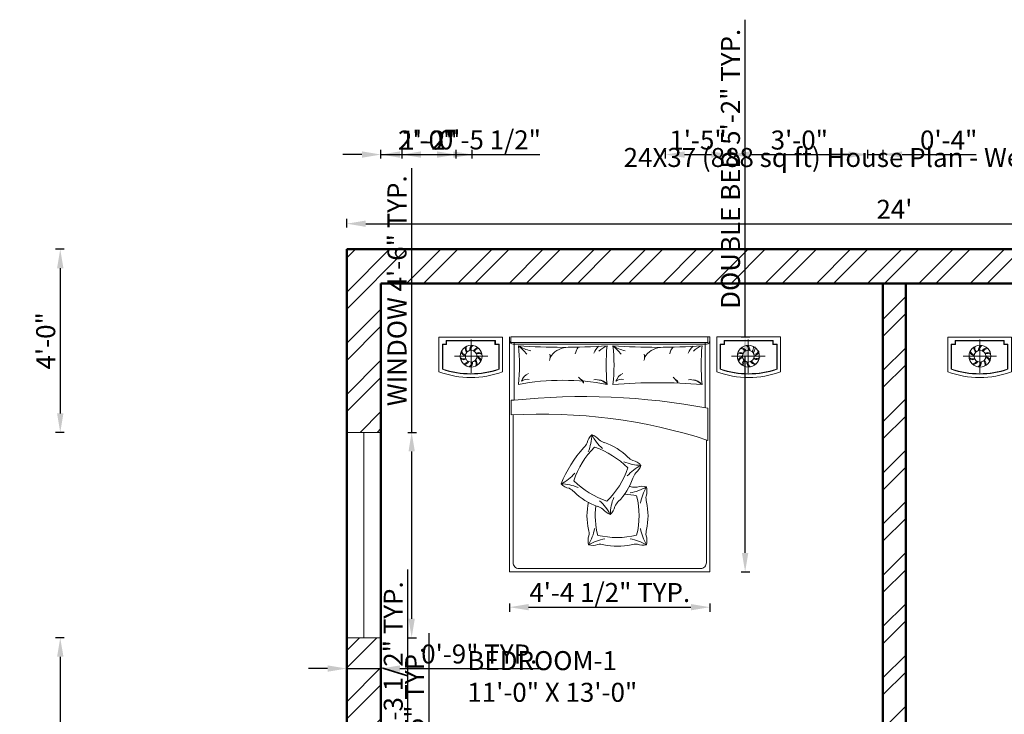
# Model space of a CAD drawing. Units: inches. Extents: x -83 to 371, y -457 to 76.
# Tile 3 of 4: x -83 to 176, y -107 to 76. Entities that reach past the tile are written whole.
import ezdxf

# ---------------------------------------------------------------- set-up
doc = ezdxf.new("R2010")
doc.units = ezdxf.units.IN
for name, color, linetype, lineweight in [('A-ANNO-DIMS', 2, 'Continuous', 18), ('A-ANNO-TEXT', 7, 'Continuous', 25), ('A-AREA-IDEN', 7, 'Continuous', 25), ('A-GLAZ', 4, 'Continuous', 18), ('A-WALL', 7, 'Continuous', 50), ('A-WALL-PATT', 252, 'Continuous', 13), ('furn', 28, 'Continuous', 18)]:
    doc.layers.add(name, color=color, linetype=linetype, lineweight=lineweight)
doc.styles.get("Standard").update_dxf_attribs({"font": 'arial.ttf'})
doc.dimstyles.new('ISO-25', dxfattribs={"dimtxt": 5, "dimasz": 5, "dimexe": 1.25, "dimexo": 0.625, "dimtad": 1, "dimlunit": 3, "dimtxsty": 'Standard', "dimcen": 2.5, "dimadec": 0, "dimazin": 0, "dimtfac": 1, "dimtmove": 0, "dimatfit": 3, "dimfxl": 1, "dimfxlon": 1, "dimarcsym": 0})

# ---------------------------------------------------------------- blocks, each defined once
blk = doc.blocks.new('*D8')
at = {"layer": 'A-ANNO-DIMS', "color": 0, "lineweight": -2, "transparency": 16777216}
for p, q in [((2.97, 21.4), (2.97, 23.65)), ((290.97, 21.4), (290.97, 23.65)), ((7.97, 22.4), (285.97, 22.4))]:
    blk.add_line(p, q, dxfattribs=at)
at = {"layer": 'A-ANNO-DIMS', "color": 0, "transparency": 16777216}
for points in [[(7.97, 23.23), (7.97, 21.56), (2.97, 22.4)], [(285.97, 23.23), (285.97, 21.56), (290.97, 22.4)]]:
    blk.add_solid(points, dxfattribs=at)
at = {"layer": 'Defpoints', "color": 0, "transparency": 16777216}
for p in [(290.97, 22.4), (2.97, 15.68), (290.97, 15.68)]:
    blk.add_point(p, dxfattribs=at)
at = {"layer": 'A-ANNO-DIMS', "color": 0, "transparency": 16777216, "insert": (146.97, 25.53), "char_height": 5, "attachment_point": 5}
blk.add_mtext("24'", dxfattribs=at)
blk = doc.blocks.new('BED-DOUBLE')
for p, q in [((0.91, 59.91), (51.75, 59.91)), ((1.17, 60.37), (1.17, 45.16)), ((51.46, 60.37), (51.46, 43.19))]:
    blk.add_line(p, q)
for points in [[(0, 61.8), (0, 0), (52.66, 0), (52.66, 61.8)], [(52.17, 61.8), (52.17, 60.37), (0.3, 60.37), (0.3, 61.8), (52.66, 61.8)]]:
    blk.add_lwpolyline(points)
for points in [[(2.33, 49.32, 0.058596), (2.33, 59.5, 0.036889), (25.64, 59.5, 0.052163), (25.64, 49.32, 0.093111)], [(27.16, 49.32, 0.058596), (27.16, 59.5, 0.036648), (50.62, 59.5, 0.052163), (50.62, 49.32, 0.036967)], [(0.46, 45.16), (1.17, 45.16, -0.072944), (52.17, 43.04), (52.17, 34.6, 0.092568), (0.46, 41.29)]]:
    blk.add_lwpolyline(points, format="xyb", close=True)
for points in [[(0.91, 41.32), (0.91, 2.43, 0.414214), (2.43, 0.91), (50.23, 0.91, 0.414214), (51.75, 2.43), (51.75, 34.75)], [(20.68, 31.62, 0.091296), (21.61, 36.08, 0.091296), (24.41, 32.49, 0.091296)], [(16.91, 24, 0.111006), (25.6, 18.59, 0.119549), (31.09, 27.39, 0.107813), (22.42, 32.82)], [(22.37, 32.81, 0.121865), (16.91, 24, 0.121865)], [(30.07, 28.97, 0.091296), (34.52, 28.03, 0.091296), (30.93, 25.24, 0.091296)], [(18.01, 22.22, 0.091296), (13.56, 23.16, 0.091296), (17.15, 25.96, 0.091296)], [(26.47, 15.11, 0.159461), (27.65, 17.2, -0.076283), (28.59, 18.51, 0.115075), (32.41, 24.64, -0.076283), (33.17, 26.05, 0.159461), (34.52, 28.03)], [(31.71, 20.79, 0.091296), (35.99, 22.35, 0.091296), (34.42, 18.08, 0.091296)], [(35.99, 7.13, 0.159461), (35.88, 9.53, -0.076283), (35.99, 11.13, 0.115075), (35.99, 18.36, -0.076283), (35.88, 19.96, 0.159461), (35.99, 22.35)], [(23.17, 9.62, 0.111006), (33.41, 9.63, 0.119549), (33.41, 19.99, 0.033212), (30.26, 20.47)], [(27.4, 19.57, 0.091296), (26.47, 15.11, 0.091296), (23.67, 18.7)], [(25.05, 8.69, 0.091296), (20.77, 7.13, 0.091296), (22.34, 11.41, 0.091296)], [(34.42, 11.41, 0.091296), (35.99, 7.13, 0.091296), (31.71, 8.69)]]:
    blk.add_lwpolyline(points, format="xyb")
for centre, radius, start, end in [((0.91, 60.83), 0.913, 180, 270), ((51.75, 60.83), 0.913, 270, 0), ((7.74, 68), 10.08, 237.5379, 257.5233), ((-5.29, 49.98), 12.19, 36.4935, 51.2792), ((8.15, 56.6), 2.53, 335.8927, 16.1192), ((15.48, 53.46), 5.64, 96.6849, 148.3182), ((21.18, 56.67), 3.96, 141.8174, 169.8987), ((26.19, 56.11), 4.26, 130.5354, 160.3558), ((28.84, 52.52), 7.67, 114.6457, 134.1585), ((19.53, 49.98), 12.19, 36.4935, 51.2792), ((32.57, 68), 10.08, 237.5379, 257.5233), ((32.98, 56.6), 2.53, 335.8927, 16.1192), ((40.3, 53.46), 5.64, 96.6849, 148.3182), ((46.01, 56.67), 3.96, 141.8174, 169.8987), ((51.01, 56.11), 4.26, 130.5354, 160.3558), ((53.67, 52.52), 7.67, 114.6457, 134.1585), ((6.34, 49.09), 3.38, 114.2916, 160.9896), ((31.17, 49.09), 3.38, 114.2916, 160.9896), ((4.59, 48.38), 2.31, 76.4823, 128.5563), ((9.19, 42.25), 12.71, 36.2085, 45.0849), ((18.6, 49.75), 0.853, 353.7543, 77.2187), ((22.67, 46.41), 4.16, 44.406, 96.8342), ((23.45, 47.86), 2.64, 33.6349, 90.8456), ((29.41, 48.38), 2.31, 76.4823, 128.5563), ((34.02, 42.25), 12.71, 36.2085, 45.0849), ((43.42, 49.75), 0.853, 353.7543, 77.2187), ((47.5, 46.41), 4.16, 44.406, 96.8342), ((48.27, 47.86), 2.64, 33.6349, 90.8456), ((15.72, 36.39), 5.29, 315.5854, 333.0343), ((24.21, 33.23), 3.86, 132.4658, 168.7065), ((20.58, 32.5), 3.72, 37.2937, 74.0973), ((26.71, 38.99), 5.29, 233.2983, 250.7472), ((19.89, 18.93), 15.91, 45.1307, 71.3884), ((44.41, 10.55), 33.33, 138.3818, 157.7644), ((34.79, 33.99), 5.29, 225.7718, 243.2208), ((31.77, 25.77), 3.56, 39.4726, 79.6505), ((16.39, 25.78), 3.86, 222.6522, 258.8929), ((13.27, 17.27), 5.29, 45.7718, 63.2208), ((28.18, 32.33), 15.91, 225.1307, 251.3884), ((28.38, 6.89), 15.91, 77.0576, 78.7033), ((33.07, 27.55), 5.29, 257.6988, 275.1477), ((34.85, 18.98), 3.56, 71.3996, 111.5774), ((36.26, 14.74), 15.91, 166.8711, 193.1289), ((44.1, 14.85), 21.58, 173.1956, 194.0284), ((21.36, 12.27), 5.29, 53.2983, 70.7472), ((27.96, 19.27), 4.41, 218.7754, 250.3571), ((15.61, 9.99), 5.29, 355.0387, 12.4877), ((24.48, 8.17), 3.86, 159.3666, 195.6073), ((21.79, 10.85), 3.86, 254.5791, 290.8198), ((23.64, 1.98), 5.29, 77.6988, 95.1477), ((28.33, 22.65), 15.91, 257.0576, 283.3153), ((33.15, 2.01), 5.29, 85.2252, 102.6741), ((35.05, 11.45), 4.41, 250.7023, 282.284)]:
    blk.add_arc(centre, radius, start, end)
blk = doc.blocks.new('NIGHTSTAND-L')
for p, q in [((8.46, 1.22), (8.46, 10)), ((4.07, 5.61), (12.85, 5.61))]:
    blk.add_line(p, q)
blk.add_lwpolyline([(0, 1.52), (0, 10.65), (16.74, 10.65), (16.74, 1.52, -0.181818)], format="xyb", close=True)
for points in [[(1.92, 9.74), (1.92, 8.74), (0.91, 8.74)], [(2.01, 9.74), (2.01, 8.65), (0.91, 8.65)], [(1.92, 9.74), (14.83, 9.74)], [(1.92, 9.65), (14.83, 9.65)], [(14.73, 9.74), (14.73, 8.65), (15.83, 8.65)], [(14.83, 9.74), (14.83, 8.74), (15.83, 8.74)]]:
    blk.add_lwpolyline(points)
for points in [[(15.83, 8.74), (15.83, 2.16, -0.167087), (0.91, 2.16), (0.91, 8.74)], [(15.74, 8.74), (15.74, 2.22, -0.165559), (1, 2.22), (1, 8.74)]]:
    blk.add_lwpolyline(points, format="xyb")
for radius in [2.87, 1.55]:
    blk.add_circle((8.46, 5.61), radius)
for centre, radius, start, end in [((8.71, 7.76), 1.84, 172.17, 218.4897), ((8.53, 7.72), 1.41, 160.3002, 220.538), ((9.93, 7.2), 1.84, 136.17, 182.4897), ((9.76, 7.27), 1.41, 124.3002, 184.538), ((10.58, 6.04), 1.84, 100.17, 146.4897), ((6.48, 6.34), 1.41, 232.3002, 292.538), ((7.4, 7.5), 1.84, 208.17, 254.4897), ((7.28, 7.36), 1.41, 196.3002, 256.538), ((10.49, 6.19), 1.41, 88.3002, 148.538), ((10.42, 4.71), 1.84, 64.17, 110.4897), ((10.44, 4.89), 1.41, 52.3002, 112.538), ((9.64, 3.86), 1.41, 16.3002, 76.538), ((9.52, 3.73), 1.84, 28.17, 74.4897), ((6.49, 6.52), 1.84, 244.17, 290.4897), ((6.43, 5.03), 1.41, 268.3002, 328.538), ((6.34, 5.19), 1.84, 280.17, 326.4897), ((7.16, 3.95), 1.41, 304.3002, 4.538), ((6.99, 4.02), 1.84, 316.17, 2.4897), ((8.38, 3.51), 1.41, 340.3002, 40.538), ((8.2, 3.47), 1.84, 352.17, 38.4897)]:
    blk.add_arc(centre, radius, start, end)
blk = doc.blocks.new('NIGHTSTAND-R')
for p, q in [((8.28, 1.22), (8.28, 10)), ((12.67, 5.61), (3.89, 5.61))]:
    blk.add_line(p, q)
blk.add_lwpolyline([(16.74, 1.52), (16.74, 10.65), (0, 10.65), (0, 1.52, 0.181818)], format="xyb", close=True)
for points in [[(1.92, 9.74), (1.92, 8.74), (0.91, 8.74)], [(2.01, 9.74), (2.01, 8.65), (0.91, 8.65)], [(14.82, 9.74), (1.92, 9.74)], [(14.82, 9.65), (1.92, 9.65)], [(14.73, 9.74), (14.73, 8.65), (15.83, 8.65)], [(14.82, 9.74), (14.82, 8.74), (15.83, 8.74)]]:
    blk.add_lwpolyline(points)
for points in [[(0.91, 8.74), (0.91, 2.16, 0.167087), (15.83, 2.16), (15.83, 8.74)], [(1, 8.74), (1, 2.22, 0.165559), (15.74, 2.22), (15.74, 8.74)]]:
    blk.add_lwpolyline(points, format="xyb")
for radius in [2.87, 1.55]:
    blk.add_circle((8.28, 5.61), radius)
for centre, radius, start, end in [((6.16, 6.03), 1.84, 33.5103, 79.83), ((6.99, 7.27), 1.41, 355.462, 55.6998), ((6.82, 7.2), 1.84, 357.5103, 43.83), ((8.21, 7.72), 1.41, 319.462, 19.6998), ((8.24, 7.84), 1.84, 321.5103, 7.83), ((6.3, 4.89), 1.41, 67.462, 127.6998), ((6.32, 4.7), 1.84, 69.5103, 115.83), ((7.23, 3.72), 1.84, 105.5103, 151.83), ((7.11, 3.86), 1.41, 103.462, 163.6998), ((6.26, 6.19), 1.41, 31.462, 91.6998), ((10.48, 6.41), 1.41, 247.462, 307.6998), ((9.67, 7.44), 1.41, 283.462, 343.6998), ((9.55, 7.58), 1.84, 285.5103, 331.83), ((8.54, 3.46), 1.84, 141.5103, 187.83), ((8.36, 3.5), 1.41, 139.462, 199.6998), ((9.75, 4.02), 1.84, 177.5103, 223.83), ((9.58, 3.95), 1.41, 175.462, 235.6998), ((10.41, 5.19), 1.84, 213.5103, 259.83), ((10.31, 5.03), 1.41, 211.462, 271.6998), ((10.46, 6.59), 1.84, 249.5103, 295.83)]:
    blk.add_arc(centre, radius, start, end)
blk = doc.blocks.new('WIN-54IN')
blk.add_line((4.5, 54), (4.5, 0))
blk.add_lwpolyline([(0, 54), (9, 54), (9, 0), (0, 0)], close=True)
blk = doc.blocks.new('*D18')
at = {"layer": 'A-ANNO-DIMS', "color": 0, "lineweight": -2, "transparency": 16777216}
for p, q in [((20.04, -32.5), (20.04, 37.02)), ((19.04, -32.5), (21.29, -32.5)), ((20.04, -81.5), (20.04, -37.5)), ((19.04, -86.5), (21.29, -86.5))]:
    blk.add_line(p, q, dxfattribs=at)
at = {"layer": 'A-ANNO-DIMS', "color": 0, "transparency": 16777216}
for points in [[(19.21, -37.5), (20.87, -37.5), (20.04, -32.5)], [(19.21, -81.5), (20.87, -81.5), (20.04, -86.5)]]:
    blk.add_solid(points, dxfattribs=at)
at = {"layer": 'Defpoints', "color": 0, "transparency": 16777216}
for p in [(11.94, -32.5), (20.04, -32.5), (11.94, -86.5)]:
    blk.add_point(p, dxfattribs=at)
at = {"layer": 'A-ANNO-DIMS', "color": 0, "transparency": 16777216, "insert": (16.83, 4.76), "char_height": 5, "attachment_point": 5, "rotation": 90}
blk.add_mtext('WINDOW 4\'-6" TYP.', dxfattribs=at)
blk = doc.blocks.new('*D19')
at = {"layer": 'A-ANNO-DIMS', "color": 0, "lineweight": -2, "transparency": 16777216}
for p, q in [((-2.06, -94.6), (-7.06, -94.6)), ((2.94, -93.6), (2.94, -95.85)), ((2.94, -94.6), (11.94, -94.6)), ((11.94, -93.6), (11.94, -95.85)), ((16.94, -94.6), (53.67, -94.6))]:
    blk.add_line(p, q, dxfattribs=at)
at = {"layer": 'A-ANNO-DIMS', "color": 0, "transparency": 16777216}
for points in [[(-2.06, -93.77), (-2.06, -95.43), (2.94, -94.6)], [(16.94, -93.77), (16.94, -95.43), (11.94, -94.6)]]:
    blk.add_solid(points, dxfattribs=at)
at = {"layer": 'Defpoints', "color": 0, "transparency": 16777216}
for p in [(2.94, -86.5), (11.94, -86.5), (11.94, -94.6)]:
    blk.add_point(p, dxfattribs=at)
at = {"layer": 'A-ANNO-DIMS', "color": 0, "transparency": 16777216, "insert": (37.8, -91.42), "char_height": 5, "attachment_point": 5}
blk.add_mtext('0\'-9" TYP.', dxfattribs=at)
blk = doc.blocks.new('*D22')
at = {"layer": 'A-ANNO-DIMS', "color": 0, "lineweight": -2, "transparency": 16777216}
for p, q in [((107.72, -7.39), (107.72, 76.05)), ((106.72, -7.39), (108.97, -7.39)), ((107.72, -64.19), (107.72, -12.39)), ((106.72, -69.19), (108.97, -69.19))]:
    blk.add_line(p, q, dxfattribs=at)
at = {"layer": 'A-ANNO-DIMS', "color": 0, "transparency": 16777216}
for points in [[(106.88, -12.39), (108.55, -12.39), (107.72, -7.39)], [(106.88, -64.19), (108.55, -64.19), (107.72, -69.19)]]:
    blk.add_solid(points, dxfattribs=at)
at = {"layer": 'Defpoints', "color": 0, "transparency": 16777216}
for p in [(98.45, -7.39), (107.72, -7.39), (98.45, -69.19)]:
    blk.add_point(p, dxfattribs=at)
at = {"layer": 'A-ANNO-DIMS', "color": 0, "transparency": 16777216, "insert": (104.51, 36.83), "char_height": 5, "attachment_point": 5, "rotation": 90}
blk.add_mtext('DOUBLE BED 5\'-2" TYP.', dxfattribs=at)
blk = doc.blocks.new('*D23')
at = {"layer": 'A-ANNO-DIMS', "color": 0, "lineweight": -2, "transparency": 16777216}
for p, q in [((45.78, -77.46), (45.78, -79.71)), ((98.45, -77.46), (98.45, -79.71)), ((50.78, -78.46), (93.45, -78.46))]:
    blk.add_line(p, q, dxfattribs=at)
at = {"layer": 'A-ANNO-DIMS', "color": 0, "transparency": 16777216}
for points in [[(50.78, -77.63), (50.78, -79.29), (45.78, -78.46)], [(93.45, -77.63), (93.45, -79.29), (98.45, -78.46)]]:
    blk.add_solid(points, dxfattribs=at)
at = {"layer": 'Defpoints', "color": 0, "transparency": 16777216}
for p in [(45.78, -69.19), (98.45, -69.19), (98.45, -78.46)]:
    blk.add_point(p, dxfattribs=at)
at = {"layer": 'A-ANNO-DIMS', "color": 0, "transparency": 16777216, "insert": (72.12, -75.25), "char_height": 5, "attachment_point": 5}
blk.add_mtext('4\'-4 1/2" TYP.', dxfattribs=at)
blk = doc.blocks.new('*D30')
at = {"layer": 'A-ANNO-DIMS', "color": 0, "lineweight": -2, "transparency": 16777216}
for p, q in [((24.67, -178.88), (24.67, -85.32)), ((24.53, -183.88), (25.92, -183.88)), ((24.67, -188.98), (24.67, -183.88)), ((24.53, -188.98), (25.92, -188.98)), ((24.67, -193.98), (24.67, -198.98))]:
    blk.add_line(p, q, dxfattribs=at)
at = {"layer": 'A-ANNO-DIMS', "color": 0, "transparency": 16777216}
for points in [[(23.83, -178.88), (25.5, -178.88), (24.67, -183.88)], [(23.83, -193.98), (25.5, -193.98), (24.67, -188.98)]]:
    blk.add_solid(points, dxfattribs=at)
at = {"layer": 'Defpoints', "color": 0, "transparency": 16777216}
for p in [(23.9, -183.88), (24.67, -183.88), (23.9, -188.98)]:
    blk.add_point(p, dxfattribs=at)
at = {"layer": 'A-ANNO-DIMS', "color": 0, "transparency": 16777216, "insert": (21.46, -129.6), "char_height": 5, "attachment_point": 5, "rotation": 90}
blk.add_mtext('LARGE BURNER 0\'-5" TYP.', dxfattribs=at)
blk = doc.blocks.new('*D32')
at = {"layer": 'A-ANNO-DIMS', "color": 0, "lineweight": -2, "transparency": 16777216}
for p, q in [((19.06, -173.23), (19.06, -68.59)), ((19.06, -178.23), (17.81, -178.23)), ((19.06, -181.8), (19.06, -178.23)), ((19.06, -181.8), (17.81, -181.8)), ((19.06, -186.8), (19.06, -191.8))]:
    blk.add_line(p, q, dxfattribs=at)
at = {"layer": 'A-ANNO-DIMS', "color": 0, "transparency": 16777216}
for points in [[(18.23, -173.23), (19.9, -173.23), (19.06, -178.23)], [(18.23, -186.8), (19.9, -186.8), (19.06, -181.8)]]:
    blk.add_solid(points, dxfattribs=at)
at = {"layer": 'Defpoints', "color": 0, "transparency": 16777216}
for p in [(19.06, -178.23), (19.6, -178.23), (19.6, -181.8)]:
    blk.add_point(p, dxfattribs=at)
at = {"layer": 'A-ANNO-DIMS', "color": 0, "transparency": 16777216, "insert": (15.85, -118.41), "char_height": 5, "attachment_point": 5, "rotation": 90}
blk.add_mtext('SMALL BURNER 0\'-3 1/2" TYP.', dxfattribs=at)
blk = doc.blocks.new('*D38')
at = {"layer": 'A-ANNO-DIMS', "color": 0, "lineweight": -2, "transparency": 16777216}
for p, q in [((-71.36, 15.68), (-73.61, 15.68)), ((-72.36, 10.68), (-72.36, -27.5)), ((-71.36, -32.5), (-73.61, -32.5))]:
    blk.add_line(p, q, dxfattribs=at)
at = {"layer": 'A-ANNO-DIMS', "color": 0, "transparency": 16777216}
for points in [[(-73.19, 10.68), (-71.52, 10.68), (-72.36, 15.68)], [(-73.19, -27.5), (-71.52, -27.5), (-72.36, -32.5)]]:
    blk.add_solid(points, dxfattribs=at)
at = {"layer": 'Defpoints', "color": 0, "transparency": 16777216}
for p in [(2.97, 15.68), (-72.36, -32.5), (2.94, -32.5)]:
    blk.add_point(p, dxfattribs=at)
at = {"layer": 'A-ANNO-DIMS', "color": 0, "transparency": 16777216, "insert": (-75.54, -8.41), "char_height": 5, "attachment_point": 5, "rotation": 90}
blk.add_mtext('4\'-0"', dxfattribs=at)
blk = doc.blocks.new('*D39')
at = {"layer": 'A-ANNO-DIMS', "color": 0, "lineweight": -2, "transparency": 16777216}
for p, q in [((-71.36, -86.5), (-73.61, -86.5)), ((-72.36, -91.5), (-72.36, -163.99)), ((-71.36, -168.99), (-73.61, -168.99))]:
    blk.add_line(p, q, dxfattribs=at)
at = {"layer": 'A-ANNO-DIMS', "color": 0, "transparency": 16777216}
for points in [[(-73.19, -91.5), (-71.52, -91.5), (-72.36, -86.5)], [(-73.19, -163.99), (-71.52, -163.99), (-72.36, -168.99)]]:
    blk.add_solid(points, dxfattribs=at)
at = {"layer": 'Defpoints', "color": 0, "transparency": 16777216}
for p in [(2.94, -86.5), (-72.36, -168.99), (3.06, -168.99)]:
    blk.add_point(p, dxfattribs=at)
at = {"layer": 'A-ANNO-DIMS', "color": 0, "transparency": 16777216, "insert": (-75.57, -127.74), "char_height": 5, "attachment_point": 5, "rotation": 90}
blk.add_mtext('6\'-10 1/2"', dxfattribs=at)
blk = doc.blocks.new('*D45')
at = {"layer": 'A-ANNO-DIMS', "color": 0, "lineweight": -2, "transparency": 16777216}
for p, q in [((143.97, -455.2), (143.97, -457.45)), ((149.97, -455.2), (149.97, -457.45)), ((138.97, -456.2), (133.97, -456.2)), ((143.97, -456.2), (149.97, -456.2)), ((154.97, -456.2), (174.51, -456.2))]:
    blk.add_line(p, q, dxfattribs=at)
at = {"layer": 'A-ANNO-DIMS', "color": 0, "transparency": 16777216}
for points in [[(138.97, -455.37), (138.97, -457.03), (143.97, -456.2)], [(154.97, -455.37), (154.97, -457.03), (149.97, -456.2)]]:
    blk.add_solid(points, dxfattribs=at)
at = {"layer": 'Defpoints', "color": 0, "transparency": 16777216}
for p in [(143.97, 6.68), (149.97, 6.68), (149.97, -456.2)]:
    blk.add_point(p, dxfattribs=at)
at = {"layer": 'A-ANNO-DIMS', "color": 0, "transparency": 16777216, "insert": (167.24, -453.02), "char_height": 5, "attachment_point": 5}
blk.add_mtext('0\'-6"', dxfattribs=at)
blk = doc.blocks.new('*D46')
at = {"layer": 'A-ANNO-DIMS', "color": 0, "lineweight": -2, "transparency": 16777216}
for p, q in [((103.97, 39.58), (103.97, 41.83)), ((139.97, 39.58), (139.97, 41.83)), ((108.97, 40.58), (134.97, 40.58))]:
    blk.add_line(p, q, dxfattribs=at)
at = {"layer": 'A-ANNO-DIMS', "color": 0, "transparency": 16777216}
for points in [[(108.97, 41.41), (108.97, 39.74), (103.97, 40.58)], [(134.97, 41.41), (134.97, 39.74), (139.97, 40.58)]]:
    blk.add_solid(points, dxfattribs=at)
at = {"layer": 'Defpoints', "color": 0, "transparency": 16777216}
for p in [(139.97, 40.58), (103.97, -149.32), (139.97, -149.32)]:
    blk.add_point(p, dxfattribs=at)
at = {"layer": 'A-ANNO-DIMS', "color": 0, "transparency": 16777216, "insert": (121.97, 43.75), "char_height": 5, "attachment_point": 5}
blk.add_mtext('3\'-0"', dxfattribs=at)
blk = doc.blocks.new('*D47')
at = {"layer": 'A-ANNO-DIMS', "color": 0, "lineweight": -2, "transparency": 16777216}
for p, q in [((139.97, 39.58), (139.97, 41.83)), ((143.97, 39.58), (143.97, 41.83)), ((134.97, 40.58), (129.97, 40.58)), ((139.97, 40.58), (143.97, 40.58)), ((148.97, 40.58), (168.51, 40.58))]:
    blk.add_line(p, q, dxfattribs=at)
at = {"layer": 'A-ANNO-DIMS', "color": 0, "transparency": 16777216}
for points in [[(134.97, 41.41), (134.97, 39.74), (139.97, 40.58)], [(148.97, 41.41), (148.97, 39.74), (143.97, 40.58)]]:
    blk.add_solid(points, dxfattribs=at)
at = {"layer": 'Defpoints', "color": 0, "transparency": 16777216}
for p in [(143.97, 40.58), (139.97, -149.32), (143.97, -149.32)]:
    blk.add_point(p, dxfattribs=at)
at = {"layer": 'A-ANNO-DIMS', "color": 0, "transparency": 16777216, "insert": (161.24, 43.75), "char_height": 5, "attachment_point": 5}
blk.add_mtext('0\'-4"', dxfattribs=at)
blk = doc.blocks.new('*D58')
at = {"layer": 'A-ANNO-DIMS', "color": 0, "lineweight": -2, "transparency": 16777216}
for p, q in [((11.97, 39.58), (11.97, 41.83)), ((35.97, 39.58), (35.97, 41.83)), ((16.97, 40.58), (30.97, 40.58))]:
    blk.add_line(p, q, dxfattribs=at)
at = {"layer": 'A-ANNO-DIMS', "color": 0, "transparency": 16777216}
for points in [[(16.97, 41.41), (16.97, 39.74), (11.97, 40.58)], [(30.97, 41.41), (30.97, 39.74), (35.97, 40.58)]]:
    blk.add_solid(points, dxfattribs=at)
at = {"layer": 'Defpoints', "color": 0, "transparency": 16777216}
for p in [(35.97, 40.58), (11.97, -155.32), (35.97, -155.32)]:
    blk.add_point(p, dxfattribs=at)
at = {"layer": 'A-ANNO-DIMS', "color": 0, "transparency": 16777216, "insert": (23.97, 43.75), "char_height": 5, "attachment_point": 5}
blk.add_mtext('2\'-0"', dxfattribs=at)
blk = doc.blocks.new('*D59')
at = {"layer": 'A-ANNO-DIMS', "color": 0, "lineweight": -2, "transparency": 16777216}
for p, q in [((17.51, 39.58), (17.51, 41.83)), ((31.73, 39.58), (31.73, 41.83)), ((22.51, 40.58), (26.73, 40.58))]:
    blk.add_line(p, q, dxfattribs=at)
at = {"layer": 'A-ANNO-DIMS', "color": 0, "transparency": 16777216}
for points in [[(22.51, 41.41), (22.51, 39.74), (17.51, 40.58)], [(26.73, 41.41), (26.73, 39.74), (31.73, 40.58)]]:
    blk.add_solid(points, dxfattribs=at)
at = {"layer": 'Defpoints', "color": 0, "transparency": 16777216}
for p in [(31.73, 40.58), (17.51, -176.2), (31.73, -176.2)]:
    blk.add_point(p, dxfattribs=at)
at = {"layer": 'A-ANNO-DIMS', "color": 0, "transparency": 16777216, "insert": (24.62, 43.71), "char_height": 5, "attachment_point": 5}
blk.add_mtext('1\'-2"', dxfattribs=at)
blk = doc.blocks.new('*D65')
at = {"layer": 'A-ANNO-DIMS', "color": 0, "lineweight": -2, "transparency": 16777216}
for p, q in [((86.8, 39.58), (86.8, 41.83)), ((103.87, 39.58), (103.87, 41.83)), ((91.8, 40.58), (98.87, 40.58))]:
    blk.add_line(p, q, dxfattribs=at)
at = {"layer": 'A-ANNO-DIMS', "color": 0, "transparency": 16777216}
for points in [[(91.8, 41.41), (91.8, 39.74), (86.8, 40.58)], [(98.87, 41.41), (98.87, 39.74), (103.87, 40.58)]]:
    blk.add_solid(points, dxfattribs=at)
at = {"layer": 'Defpoints', "color": 0, "transparency": 16777216}
for p in [(103.87, 40.58), (103.87, -209.32), (86.8, -211.22)]:
    blk.add_point(p, dxfattribs=at)
at = {"layer": 'A-ANNO-DIMS', "color": 0, "transparency": 16777216, "insert": (95.33, 43.75), "char_height": 5, "attachment_point": 5}
blk.add_mtext('1\'-5"', dxfattribs=at)
blk = doc.blocks.new('*D67')
at = {"layer": 'A-ANNO-DIMS', "color": 0, "lineweight": -2, "transparency": 16777216}
for p, q in [((11.97, 39.58), (11.97, 41.83)), ((17.51, 39.58), (17.51, 41.83)), ((6.97, 40.58), (1.97, 40.58)), ((11.97, 40.58), (17.51, 40.58)), ((22.51, 40.58), (53.7, 40.58))]:
    blk.add_line(p, q, dxfattribs=at)
at = {"layer": 'A-ANNO-DIMS', "color": 0, "transparency": 16777216}
for points in [[(6.97, 41.41), (6.97, 39.74), (11.97, 40.58)], [(22.51, 41.41), (22.51, 39.74), (17.51, 40.58)]]:
    blk.add_solid(points, dxfattribs=at)
at = {"layer": 'Defpoints', "color": 0, "transparency": 16777216}
for p in [(17.51, 40.58), (11.97, -155.32), (17.51, -176.2)]:
    blk.add_point(p, dxfattribs=at)
at = {"layer": 'A-ANNO-DIMS', "color": 0, "transparency": 16777216, "insert": (40.61, 43.79), "char_height": 5, "attachment_point": 5}
blk.add_mtext('0\'-5 1/2"', dxfattribs=at)

msp = doc.modelspace()

# ---------------------------------------------------------------- hatches: boundary and pattern name
at = {"layer": 'A-WALL-PATT'}
h = msp.add_hatch(dxfattribs=at)
h.set_pattern_fill('ANSI32', color=256)
h.set_pattern_definition([(45, (-445.966, 5e-14), (-6.73519, 6.73519), []), (45, (-441.476, 5e-14), (-6.73519, 6.73519), [])])
h.paths.add_polyline_path([(147.969, -419.325), (11.969, -419.325), (11.969, -408.128), (2.969, -408.128), (2.969, -428.325), (147.969, -428.325)])
h.paths.add_polyline_path([(290.969, -408.128), (281.969, -408.128), (281.969, -419.325), (197.969, -419.325), (197.969, -428.325), (290.969, -428.325)])
h.paths.add_polyline_path([(203.969, -374.325), (207.969, -374.325), (207.969, -368.325), (203.969, -368.325), (203.969, -279.294), (197.969, -279.294), (197.969, -317.37), (194.142, -317.37), (194.142, -317.678), (194.142, -323.37), (197.969, -323.37), (197.969, -374.325), (197.969, -419.325), (203.969, -419.325)])
h.paths.add_polyline_path([(290.969, -249.793), (281.969, -249.793), (281.969, -390.128), (290.969, -390.128)])
h.paths.add_polyline_path([(149.969, -323.37), (157.969, -323.37), (157.969, -317.37), (149.969, -317.37), (149.969, -279.294), (143.969, -279.294), (143.969, -371.325), (140.142, -371.325), (140.142, -371.632), (140.142, -377.325), (143.969, -377.325), (149.969, -377.325)])
h.paths.add_polyline_path([(103.969, -371.325), (11.969, -371.325), (11.969, -377.325), (103.969, -377.325)])
h.paths.add_polyline_path([(11.969, -328.391), (3.855, -328.391), (3.855, -274.391), (11.969, -274.391), (11.969, -222.986), (2.969, -222.986), (2.969, -390.128), (11.969, -390.128)])
h.paths.add_polyline_path([(149.969, -233.325), (143.969, -233.325), (11.969, -233.325), (11.969, -239.325), (143.969, -239.325), (143.969, -243.294), (144.688, -243.294), (149.969, -243.294)])
h.paths.add_polyline_path([(11.969, -86.501), (2.969, -86.501), (2.969, -168.986), (11.969, -168.986)])
h.paths.add_polyline_path([(103.969, -149.325), (11.969, -149.325), (11.969, -155.325), (103.969, -155.325)])
h.paths.add_polyline_path([(149.969, 6.675), (143.969, 6.675), (143.969, -149.325), (139.969, -149.325), (139.969, -155.325), (153.969, -155.325), (153.969, -149.325), (149.969, -149.325)])
h.paths.add_polyline_path([(281.969, -149.325), (189.973, -149.325, -0.0041567), (189.978, -149.923), (189.978, -155.325), (281.969, -155.325)])
h.paths.add_polyline_path([(290.969, -90.886), (281.969, -90.886), (281.969, -195.793), (290.969, -195.793)])
h.paths.add_polyline_path([(290.969, 15.675), (2.969, 15.675), (2.969, -32.501), (11.969, -32.501), (11.969, 6.675), (281.969, 6.675), (281.969, -36.886), (290.969, -36.886)])

# ---------------------------------------------------------------- linework, layer by layer
at = {"layer": 'A-WALL'}
for p, q in [((2.969, 15.675), (290.969, 15.675)), ((2.969, -428.325), (2.969, 15.675)), ((11.969, 6.675), (281.969, 6.675)), ((11.969, -419.325), (11.969, 6.675)), ((143.969, -149.325), (143.969, 6.675)), ((149.969, -149.325), (149.969, 6.675))]:
    msp.add_line(p, q, dxfattribs=at)

# ---------------------------------------------------------------- block references
at = {"layer": 'A-GLAZ'}
msp.add_blockref('WIN-54IN', (2.938, -86.5), dxfattribs=at)
at = {"layer": 'furn'}
for name, p in [('NIGHTSTAND-L', (27.215, -18.053)), ('BED-DOUBLE', (45.785, -69.19)), ('NIGHTSTAND-R', (100.275, -18.05)), ('NIGHTSTAND-L', (161.006, -18.053))]:
    msp.add_blockref(name, p, dxfattribs=at)

# ---------------------------------------------------------------- texts
at = {"layer": 'A-ANNO-TEXT', "insert": (75.772, 42.316), "char_height": 5, "attachment_point": 1}
msp.add_mtext_dynamic_manual_height_columns('24X37 (888 sq ft) House Plan - West Face - FP1323', width=296.42101, gutter_width=12.5, heights=[0], dxfattribs=at)
at = {"layer": 'A-AREA-IDEN', "insert": (34.677, -90.018), "char_height": 5, "attachment_point": 1}
msp.add_mtext_dynamic_manual_height_columns('BEDROOM-1\\P11\'-0" X 13\'-0"', width=60.06618, gutter_width=12.5, heights=[0], dxfattribs=at)

# ---------------------------------------------------------------- dimensions: what is measured, and where the dimension line sits
at = {"layer": 'A-ANNO-DIMS'}
for base, p1, p2, text, picture, middle in [((107.718, -7.394), (98.448, -69.19), (98.448, -7.394), 'DOUBLE BED <> TYP.', '*D22', (104.506, 36.829)), ((20.039, -32.501), (11.939, -86.501), (11.939, -32.501), 'WINDOW <> TYP.', '*D18', (16.827, 4.76)), ((19.062, -178.232), (19.597, -181.797), (19.597, -178.232), 'SMALL BURNER <> TYP.', '*D32', (15.85, -118.413)), ((24.666, -183.882), (23.902, -188.975), (23.902, -183.882), 'LARGE BURNER <> TYP.', '*D30', (21.456, -129.601))]:
    dim = msp.add_linear_dim(base=base, p1=p1, p2=p2, angle=90, text=text, dimstyle='ISO-25', override={"dimdec": 1, "dimlfac": 1, "dimrnd": 0, "dimzin": 1, "dimdsep": 46, "dimlunit": 4, "dimfrac": 2}, dxfattribs=at)
    dim.commit()
    dim.dimension.update_dxf_attribs({"geometry": picture, "text_midpoint": middle})
for base, p1, p2, override, picture, middle in [((17.509, 40.575), (11.969, -155.325), (17.509, -176.204), {"dimdec": 1, "dimlfac": 1, "dimrnd": 0, "dimzin": 1, "dimdsep": 46, "dimlunit": 4, "dimfrac": 2}, '*D67', (40.605, 43.786)), ((35.969, 40.575), (11.969, -155.325), (35.969, -155.325), {"dimdec": 1, "dimlfac": 1, "dimrnd": 0, "dimzin": 1, "dimdsep": 46, "dimlunit": 4, "dimfrac": 2}, '*D58', (23.969, 43.753)), ((31.729, 40.575), (17.509, -176.204), (31.729, -176.204), {"dimdec": 1, "dimlfac": 1, "dimrnd": 0, "dimzin": 1, "dimdsep": 46, "dimlunit": 4, "dimfrac": 2}, '*D59', (24.619, 43.711)), ((103.866, 40.575), (86.802, -211.219), (103.866, -209.325), {"dimdec": 1, "dimlfac": 1, "dimrnd": 0, "dimzin": 1, "dimdsep": 46, "dimlunit": 4, "dimfrac": 2}, '*D65', (95.334, 43.753)), ((139.969, 40.575), (103.969, -149.325), (139.969, -149.325), {"dimdec": 1, "dimlfac": 1, "dimrnd": 0, "dimzin": 1, "dimdsep": 46, "dimlunit": 4, "dimfrac": 2}, '*D46', (121.969, 43.755)), ((143.969, 40.575), (139.969, -149.325), (143.969, -149.325), {"dimdec": 1, "dimlfac": 1, "dimrnd": 0, "dimzin": 1, "dimdsep": 46, "dimlunit": 4, "dimfrac": 2}, '*D47', (161.24, 43.753)), ((290.969, 22.396), (2.969, 15.675), (290.969, 15.675), {"dimclrd": 0, "dimclre": 0, "dimclrt": 0}, '*D8', (146.969, 25.531)), ((149.969, -456.2), (143.969, 6.675), (149.969, 6.675), {"dimdec": 1, "dimlfac": 1, "dimrnd": 0, "dimzin": 1, "dimdsep": 46, "dimlunit": 4, "dimfrac": 2}, '*D45', (167.24, -453.022))]:
    dim = msp.add_linear_dim(base=base, p1=p1, p2=p2, dimstyle='ISO-25', override=override, dxfattribs=at)
    dim.commit()
    dim.dimension.update_dxf_attribs({"geometry": picture, "text_midpoint": middle})
for base, p1, p2, picture, middle in [((-72.358, -32.501), (2.969, 15.675), (2.939, -32.501), '*D38', (-75.536, -8.413)), ((-72.358, -168.986), (2.939, -86.501), (3.062, -168.986), '*D39', (-75.568, -127.743))]:
    dim = msp.add_linear_dim(base=base, p1=p1, p2=p2, angle=90, dimstyle='ISO-25', override={"dimdec": 1, "dimlfac": 1, "dimrnd": 0, "dimzin": 1, "dimdsep": 46, "dimlunit": 4, "dimfrac": 2}, dxfattribs=at)
    dim.commit()
    dim.dimension.update_dxf_attribs({"geometry": picture, "text_midpoint": middle})
for base, p1, p2, picture, middle in [((98.448, -78.46), (45.785, -69.19), (98.448, -69.19), '*D23', (72.116, -75.249)), ((11.939, -94.601), (2.939, -86.501), (11.939, -86.501), '*D19', (37.802, -91.423))]:
    dim = msp.add_linear_dim(base=base, p1=p1, p2=p2, text='<> TYP.', dimstyle='ISO-25', override={"dimdec": 1, "dimlfac": 1, "dimrnd": 0, "dimzin": 1, "dimdsep": 46, "dimlunit": 4, "dimfrac": 2}, dxfattribs=at)
    dim.commit()
    dim.dimension.update_dxf_attribs({"geometry": picture, "text_midpoint": middle})

doc.saveas('drawing.dxf')
